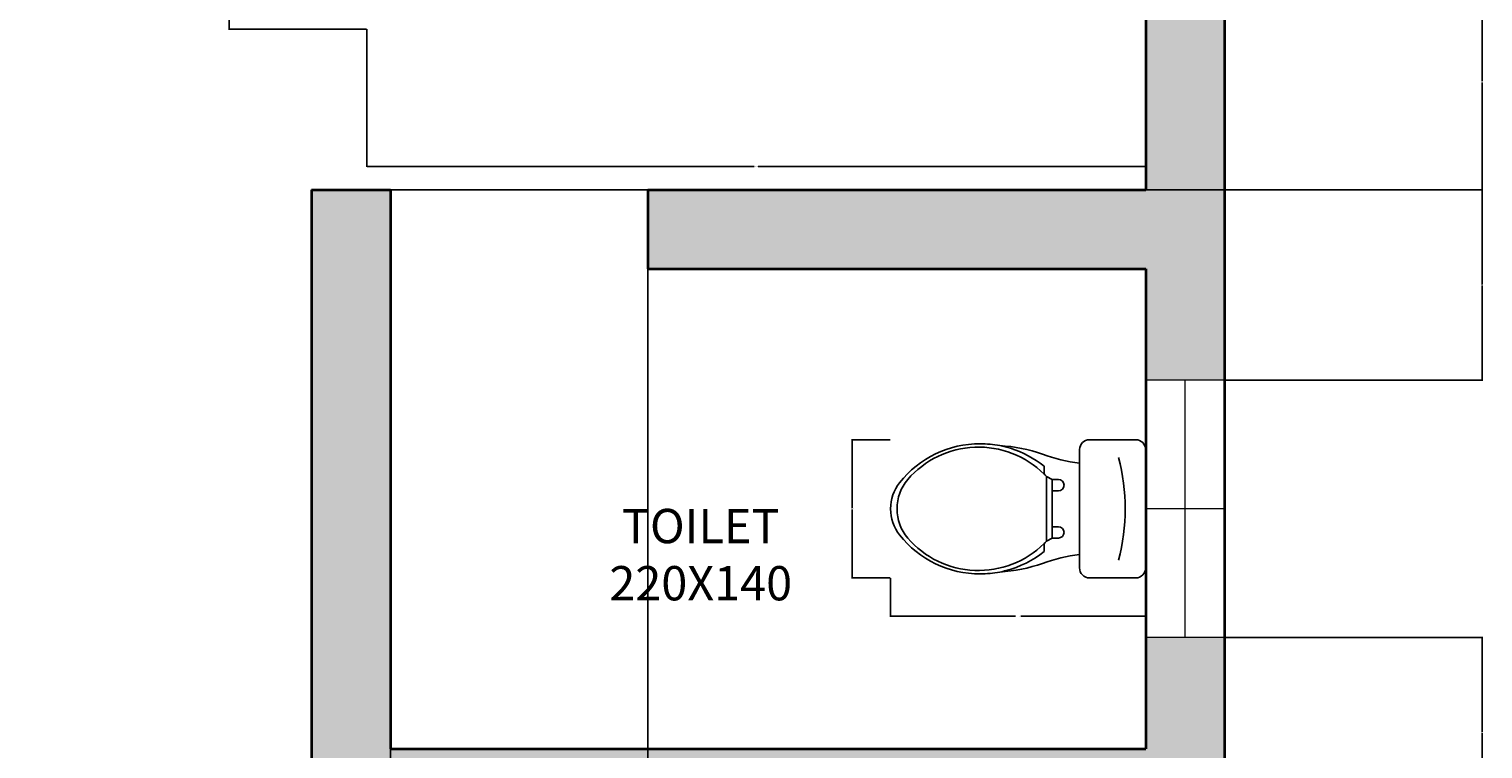
# Model space of a CAD drawing. Units: centimetres. Extents: x 2178 to 3635, y 1064 to 2635.
# Tile 7 of 9: x 3211 to 3635, y 1765 to 1974. Entities that reach past the tile are written whole.
import ezdxf

# ---------------------------------------------------------------- set-up
doc = ezdxf.new("R2010")
doc.units = ezdxf.units.CM
for name, color, linetype, lineweight in [('A-ANNO-DIMS', 2, 'Continuous', 18), ('A-AREA-IDEN', 7, 'Continuous', 18), ('A-DOOR', 32, 'Continuous', 25), ('A-FLOR-FIXT', 42, 'Continuous', 18), ('A-GLAZ', 4, 'Continuous', 18), ('A-WALL', 7, 'Continuous', 35)]:
    doc.layers.add(name, color=color, linetype=linetype, lineweight=lineweight)
doc.layers.add('A-WALL-PATT', color=18, linetype='Continuous', lineweight=13, true_color=0x000000)
doc.layers.add('WC-Detail_dwgmodels.com', color=251, linetype='Continuous')
doc.layers.add('WC-Outline_dwgmodels.com', color=250, linetype='Continuous')
doc.styles.get("Standard").update_dxf_attribs({"font": 'arial.ttf'})
doc.dimstyles.get("Standard").update_dxf_attribs({"dimtxt": 0.18, "dimasz": 0.18, "dimexe": 0.18, "dimexo": 0.0625, "dimgap": 0.09, "dimtad": 0, "dimtih": 1, "dimtoh": 1, "dimdec": 4, "dimzin": 0, "dimdsep": 46, "dimtxsty": 'Standard', "dimcen": 0.09, "dimadec": 0, "dimazin": 0, "dimtfac": 1, "dimtdec": 4, "dimtofl": 0, "dimtmove": 0, "dimatfit": 3, "dimfxl": 1, "dimtolj": 1, "dimtzin": 0, "dimarcsym": 0})

# ---------------------------------------------------------------- blocks, each defined once
blk = doc.blocks.new('pan')
at = {"layer": 'WC-Detail_dwgmodels.com'}
for p, q in [((2845.06, 2654.5), (2845.98, 2656.18)), ((2845.98, 2656.18), (2845.98, 2658.01)), ((2849.25, 2656.18), (2845.98, 2656.18)), ((2849.25, 2658.01), (2849.25, 2656.18)), ((2854.51, 2656.18), (2849.25, 2656.18)), ((2854.51, 2656.18), (2859.76, 2656.18)), ((2859.76, 2658.01), (2859.76, 2656.18)), ((2859.76, 2656.18), (2863.04, 2656.18)), ((2863.04, 2656.18), (2863.04, 2658.01)), ((2863.95, 2654.5), (2863.04, 2656.18)), ((2844.36, 2653.82), (2842.09, 2653.82)), ((2854.51, 2654.5), (2845.06, 2654.5)), ((2854.51, 2654.5), (2863.95, 2654.5)), ((2864.65, 2653.82), (2866.93, 2653.82))]:
    blk.add_line(p, q, dxfattribs=at)
for centre, radius, start, end in [((2854.54, 2618.37), 59.08, 90.028, 104.6712), ((2854.48, 2618.37), 59.08, 75.3288, 89.972), ((2847.61, 2658.01), 1.64, 0, 180), ((2861.4, 2658.01), 1.64, 0, 180), ((2863.72, 2634.72), 27.2, 135.3828, 229.2681), ((2865.36, 2635.16), 29.83, 141.274, 162.7649), ((2863.72, 2634.72), 27.2, 133.3236, 135.3828), ((2845.29, 2634.72), 27.2, 310.7319, 44.6172), ((2845.29, 2634.72), 27.2, 44.6172, 46.6764), ((2843.66, 2635.16), 29.83, 14.6482, 38.726), ((2865.36, 2635.16), 29.83, 162.7649, 168.8583), ((2843.66, 2635.16), 29.83, 11.1417, 14.6482), ((2854.36, 2623.84), 12.85, 229.2681, 270.6684), ((2854.66, 2623.84), 12.85, 269.3316, 310.7319)]:
    blk.add_arc(centre, radius, start, end, dxfattribs=at)
at = {"layer": 'WC-Outline_dwgmodels.com'}
for p, q in [((2854.51, 2683.42), (2837.26, 2683.42)), ((2871.75, 2683.42), (2854.51, 2683.42)), ((2834.37, 2680.53), (2834.37, 2667.05)), ((2874.65, 2667.05), (2874.65, 2680.53)), ((2837.26, 2664.16), (2841.21, 2664.16)), ((2841.21, 2664.16), (2854.51, 2664.16)), ((2867.8, 2664.16), (2854.51, 2664.16)), ((2867.8, 2664.16), (2871.75, 2664.16))]:
    blk.add_line(p, q, dxfattribs=at)
for centre, radius, start, end in [((2837.26, 2680.53), 2.89, 90, 180), ((2871.75, 2680.53), 2.89, 360, 90), ((2837.26, 2667.05), 2.89, 180, 270), ((2788.54, 2671.16), 53.13, 340.4442, 352.4299), ((2920.47, 2671.16), 53.13, 187.5701, 199.5558), ((2871.75, 2667.05), 2.89, 270, 0), ((2880.9, 2638.36), 44.88, 160.4442, 176.7189), ((2828.12, 2638.36), 44.88, 3.2811, 19.5558), ((2865.36, 2635.16), 29.83, 168.8583, 179.8559), ((2843.66, 2635.16), 29.83, 0.1441, 11.1417), ((2865.36, 2635.16), 29.83, 179.8559, 231.7417), ((2843.66, 2635.16), 29.83, 308.2583, 0.1441), ((2854.51, 2621.4), 12.31, 231.7417, 269.9885), ((2854.5, 2621.4), 12.31, 270.0115, 308.2583)]:
    blk.add_arc(centre, radius, start, end, dxfattribs=at)
blk = doc.blocks.new('WIN-0750-2LT')
for p, q in [((0, 0), (0, 23)), ((37.5, 0), (37.5, 23)), ((75, 0), (75, 23)), ((0, 11.5), (75, 11.5))]:
    blk.add_line(p, q)
blk = doc.blocks.new('DOOR-0750')
blk.add_line((0, 0), (75, 0))
blk = doc.blocks.new('*D28')
at = {"layer": 'A-ANNO-DIMS', "color": 0, "lineweight": -2, "transparency": 16777216}
for p, q in [((3309.61, 2241.29), (3269.47, 2241.29)), ((3269.65, 2241.11), (3269.65, 2108.05)), ((3269.65, 1974.63), (3269.65, 2107.68)), ((3309.61, 1974.45), (3269.47, 1974.45))]:
    blk.add_line(p, q, dxfattribs=at)
at = {"layer": 'A-ANNO-DIMS', "color": 0, "transparency": 16777216}
for points in [[(3269.62, 2241.11), (3269.68, 2241.11), (3269.65, 2241.29)], [(3269.62, 1974.63), (3269.68, 1974.63), (3269.65, 1974.45)]]:
    blk.add_solid(points, dxfattribs=at)
at = {"layer": 'Defpoints', "color": 0, "transparency": 16777216}
for p in [(3309.68, 2241.29), (3269.65, 1974.45), (3309.68, 1974.45)]:
    blk.add_point(p, dxfattribs=at)
at = {"layer": 'A-ANNO-DIMS', "color": 0, "transparency": 16777216, "insert": (3269.65, 2107.87), "char_height": 0.18, "attachment_point": 5}
blk.add_mtext('\\A1;BED GROUP 267 TYP.', dxfattribs=at)
blk = doc.blocks.new('*D29')
at = {"layer": 'A-ANNO-DIMS', "color": 0, "lineweight": -2, "transparency": 16777216}
for p, q in [((3309.68, 1974.38), (3309.68, 1934.24)), ((3536.6, 1974.38), (3536.6, 1934.24)), ((3309.86, 1934.42), (3422.54, 1934.42)), ((3536.42, 1934.42), (3423.74, 1934.42))]:
    blk.add_line(p, q, dxfattribs=at)
at = {"layer": 'A-ANNO-DIMS', "color": 0, "transparency": 16777216}
for points in [[(3309.86, 1934.45), (3309.86, 1934.39), (3309.68, 1934.42)], [(3536.42, 1934.45), (3536.42, 1934.39), (3536.6, 1934.42)]]:
    blk.add_solid(points, dxfattribs=at)
at = {"layer": 'Defpoints', "color": 0, "transparency": 16777216}
for p in [(3309.68, 1974.45), (3536.6, 1974.45), (3536.6, 1934.42)]:
    blk.add_point(p, dxfattribs=at)
at = {"layer": 'A-ANNO-DIMS', "color": 0, "transparency": 16777216, "insert": (3423.14, 1934.42), "char_height": 0.18, "attachment_point": 5}
blk.add_mtext('\\A1;227 TYP.', dxfattribs=at)
blk = doc.blocks.new('*D30')
at = {"layer": 'A-ANNO-DIMS', "color": 0, "lineweight": -2, "transparency": 16777216}
for p, q in [((3462.28, 1814.39), (3462.28, 1803.12)), ((3536.6, 1814.39), (3536.6, 1803.12)), ((3462.46, 1803.3), (3498.67, 1803.3)), ((3536.42, 1803.3), (3500.22, 1803.3))]:
    blk.add_line(p, q, dxfattribs=at)
at = {"layer": 'A-ANNO-DIMS', "color": 0, "transparency": 16777216}
for points in [[(3462.46, 1803.33), (3462.46, 1803.27), (3462.28, 1803.3)], [(3536.42, 1803.33), (3536.42, 1803.27), (3536.6, 1803.3)]]:
    blk.add_solid(points, dxfattribs=at)
at = {"layer": 'Defpoints', "color": 0, "transparency": 16777216}
for p in [(3462.28, 1814.45), (3536.6, 1814.45), (3536.6, 1803.3)]:
    blk.add_point(p, dxfattribs=at)
at = {"layer": 'A-ANNO-DIMS', "color": 0, "transparency": 16777216, "insert": (3499.44, 1803.3), "char_height": 0.18, "attachment_point": 5}
blk.add_mtext('\\A1;WC 74 TYP.', dxfattribs=at)
blk = doc.blocks.new('*D31')
at = {"layer": 'A-ANNO-DIMS', "color": 0, "lineweight": -2, "transparency": 16777216}
for p, q in [((3462.22, 1854.73), (3450.95, 1854.73)), ((3451.13, 1854.55), (3451.13, 1834.77)), ((3451.13, 1814.63), (3451.13, 1834.41)), ((3462.22, 1814.45), (3450.95, 1814.45))]:
    blk.add_line(p, q, dxfattribs=at)
at = {"layer": 'A-ANNO-DIMS', "color": 0, "transparency": 16777216}
for points in [[(3451.1, 1854.55), (3451.16, 1854.55), (3451.13, 1854.73)], [(3451.1, 1814.63), (3451.16, 1814.63), (3451.13, 1814.45)]]:
    blk.add_solid(points, dxfattribs=at)
at = {"layer": 'Defpoints', "color": 0, "transparency": 16777216}
for p in [(3462.28, 1854.73), (3451.13, 1814.45), (3462.28, 1814.45)]:
    blk.add_point(p, dxfattribs=at)
at = {"layer": 'A-ANNO-DIMS', "color": 0, "transparency": 16777216, "insert": (3451.13, 1834.59), "char_height": 0.18, "attachment_point": 5}
blk.add_mtext('\\A1;40 TYP.', dxfattribs=at)
blk = doc.blocks.new('*D56')
at = {"layer": 'A-ANNO-DIMS', "color": 0, "lineweight": -2, "transparency": 16777216}
for p, q in [((3559.67, 1990.59), (3634.78, 1990.59)), ((3634.6, 1990.41), (3634.6, 1959.27)), ((3634.6, 1927.77), (3634.6, 1958.91)), ((3536.67, 1927.59), (3634.78, 1927.59))]:
    blk.add_line(p, q, dxfattribs=at)
at = {"layer": 'A-ANNO-DIMS', "color": 0, "transparency": 16777216}
for points in [[(3634.57, 1990.41), (3634.63, 1990.41), (3634.6, 1990.59)], [(3634.57, 1927.77), (3634.63, 1927.77), (3634.6, 1927.59)]]:
    blk.add_solid(points, dxfattribs=at)
at = {"layer": 'Defpoints', "color": 0, "transparency": 16777216}
for p in [(3559.6, 1990.59), (3634.6, 1990.59), (3536.6, 1927.59)]:
    blk.add_point(p, dxfattribs=at)
at = {"layer": 'A-ANNO-DIMS', "color": 0, "transparency": 16777216, "insert": (3634.6, 1959.09), "char_height": 0.18, "attachment_point": 5}
blk.add_mtext('\\A1;63', dxfattribs=at)
blk = doc.blocks.new('*D57')
at = {"layer": 'A-ANNO-DIMS', "color": 0, "lineweight": -2, "transparency": 16777216}
for p, q in [((3536.67, 1927.59), (3634.78, 1927.59)), ((3634.6, 1927.41), (3634.6, 1900.02)), ((3634.6, 1872.27), (3634.6, 1899.66)), ((3559.67, 1872.09), (3634.78, 1872.09))]:
    blk.add_line(p, q, dxfattribs=at)
at = {"layer": 'A-ANNO-DIMS', "color": 0, "transparency": 16777216}
for points in [[(3634.57, 1927.41), (3634.63, 1927.41), (3634.6, 1927.59)], [(3634.57, 1872.27), (3634.63, 1872.27), (3634.6, 1872.09)]]:
    blk.add_solid(points, dxfattribs=at)
at = {"layer": 'Defpoints', "color": 0, "transparency": 16777216}
for p in [(3536.6, 1927.59), (3634.6, 1927.59), (3559.6, 1872.09)]:
    blk.add_point(p, dxfattribs=at)
at = {"layer": 'A-ANNO-DIMS', "color": 0, "transparency": 16777216, "insert": (3634.6, 1899.84), "char_height": 0.18, "attachment_point": 5}
blk.add_mtext('\\A1;55.5', dxfattribs=at)
blk = doc.blocks.new('*D58')
at = {"layer": 'A-ANNO-DIMS', "color": 0, "lineweight": -2, "transparency": 16777216}
for p, q in [((3559.67, 1797.09), (3634.78, 1797.09)), ((3634.6, 1796.91), (3634.6, 1769.52)), ((3634.6, 1741.77), (3634.6, 1769.16)), ((3559.67, 1741.59), (3634.78, 1741.59))]:
    blk.add_line(p, q, dxfattribs=at)
at = {"layer": 'A-ANNO-DIMS', "color": 0, "transparency": 16777216}
for points in [[(3634.57, 1796.91), (3634.63, 1796.91), (3634.6, 1797.09)], [(3634.57, 1741.77), (3634.63, 1741.77), (3634.6, 1741.59)]]:
    blk.add_solid(points, dxfattribs=at)
at = {"layer": 'Defpoints', "color": 0, "transparency": 16777216}
for p in [(3559.6, 1797.09), (3634.6, 1797.09), (3559.6, 1741.59)]:
    blk.add_point(p, dxfattribs=at)
at = {"layer": 'A-ANNO-DIMS', "color": 0, "transparency": 16777216, "insert": (3634.6, 1769.34), "char_height": 0.18, "attachment_point": 5}
blk.add_mtext('\\A1;55.5', dxfattribs=at)
blk = doc.blocks.new('*D67')
at = {"layer": 'A-ANNO-DIMS', "color": 0, "lineweight": -2, "transparency": 16777216}
for p, q in [((3316.6, 1927.53), (3316.6, 1113.41)), ((3391.6, 1927.53), (3391.6, 1113.41)), ((3316.78, 1113.59), (3353.89, 1113.59)), ((3391.42, 1113.59), (3354.32, 1113.59))]:
    blk.add_line(p, q, dxfattribs=at)
at = {"layer": 'A-ANNO-DIMS', "color": 0, "transparency": 16777216}
for points in [[(3316.78, 1113.62), (3316.78, 1113.56), (3316.6, 1113.59)], [(3391.42, 1113.62), (3391.42, 1113.56), (3391.6, 1113.59)]]:
    blk.add_solid(points, dxfattribs=at)
at = {"layer": 'Defpoints', "color": 0, "transparency": 16777216}
for p in [(3316.6, 1927.59), (3391.6, 1927.59), (3391.6, 1113.59)]:
    blk.add_point(p, dxfattribs=at)
at = {"layer": 'A-ANNO-DIMS', "color": 0, "transparency": 16777216, "insert": (3354.1, 1113.59), "char_height": 0.18, "attachment_point": 5}
blk.add_mtext('\\A1;75', dxfattribs=at)

msp = doc.modelspace()

# ---------------------------------------------------------------- hatches: boundary and pattern name
at = {"layer": 'A-WALL-PATT'}
h = msp.add_hatch(color=256, dxfattribs=at)
h.dxf.hatch_style = 1
h.paths.add_polyline_path([(2276.605, 2499.59), (2253.605, 2499.59), (2253.605, 2476.59), (2276.605, 2476.59)])
h.paths.add_polyline_path([(2411.605, 2350.59), (2253.605, 2350.59), (2253.605, 2327.59), (2411.605, 2327.59)])
h.paths.add_polyline_path([(2276.605, 2252.59), (2253.605, 2252.59), (2253.605, 2020.59), (2276.605, 2020.59), (2276.605, 2093.59), (2561.605, 2093.59), (2561.605, 2116.59), (2276.605, 2116.59)])
h.paths.add_polyline_path([(2659.605, 1787.59), (2610.616, 1787.59), (2276.605, 1787.59), (2276.605, 1860.59), (2253.605, 1860.59), (2253.605, 1732.09), (2276.605, 1732.09), (2276.605, 1764.59), (2516.605, 1764.59), (2516.605, 1699.59), (2539.605, 1699.59), (2539.605, 1764.59), (2659.605, 1764.59)])
h.paths.add_polyline_path([(2539.605, 1624.59), (2276.605, 1624.59), (2276.605, 1657.09), (2253.605, 1657.09), (2253.605, 1561.59), (2276.605, 1561.59), (2276.605, 1601.59), (2539.605, 1601.59)])
h.paths.add_polyline_path([(2276.605, 1501.59), (2253.605, 1501.59), (2253.605, 1371.59), (2276.605, 1371.59)])
h.paths.add_polyline_path([(2376.605, 1271.59), (2276.605, 1271.59), (2276.605, 1311.59), (2253.605, 1311.59), (2253.605, 1248.59), (2376.605, 1248.59)])
h.paths.add_polyline_path([(2636.605, 1271.59), (2536.605, 1271.59), (2536.605, 1248.59), (2636.605, 1248.59)])
h.paths.add_polyline_path([(2659.605, 1600.59), (2919.605, 1600.59), (2919.605, 1623.59), (2636.605, 1623.59), (2636.605, 1188.59), (2659.605, 1188.59)])
h.paths.add_polyline_path([(2939.605, 1211.59), (2759.605, 1211.59), (2759.605, 1188.59), (2939.605, 1188.59)])
h.paths.add_polyline_path([(3062.605, 1288.59), (3039.605, 1288.59), (3039.605, 1188.59), (3062.605, 1188.59)])
h.paths.add_polyline_path([(3372.605, 1248.59), (3062.605, 1248.59), (3062.605, 1218.59), (3372.605, 1218.59)])
h.paths.add_polyline_path([(3395.605, 1271.59), (3372.605, 1271.59), (3372.605, 1248.59), (3395.605, 1248.59)])
h.paths.add_polyline_path([(3559.605, 1271.59), (3536.605, 1271.59), (3536.605, 1248.59), (3559.605, 1248.59)])
h.paths.add_polyline_path([(3559.605, 1623.59), (3536.605, 1623.59), (3536.605, 1600.59), (3559.605, 1600.59)])
h.paths.add_polyline_path([(3395.605, 1623.59), (3162.605, 1623.59), (3162.605, 1600.59), (3395.605, 1600.59)])
h.paths.add_polyline_path([(3395.605, 1411.59), (3277.1, 1411.59), (3277.1, 1388.59), (3395.605, 1388.59)])
h.paths.add_polyline_path([(3157.1, 1411.59), (3062.605, 1411.59), (3062.605, 1623.59), (3039.605, 1623.59), (3039.605, 1388.59), (3157.1, 1388.59)])
h.paths.add_polyline_path([(3559.605, 1797.09), (3536.605, 1797.09), (3536.605, 1764.59), (3316.605, 1764.59), (3316.605, 1927.59), (3293.605, 1927.59), (3293.605, 1741.59), (3372.605, 1741.59), (3395.605, 1741.59), (3559.605, 1741.59)])
h.paths.add_polyline_path([(3559.605, 1990.59), (3536.605, 1990.59), (3536.605, 1974.446), (3536.605, 1927.59), (3391.605, 1927.59), (3391.605, 1904.59), (3536.605, 1904.59), (3536.605, 1872.09), (3559.605, 1872.09)])
h.paths.add_polyline_path([(3559.605, 2180.59), (3536.605, 2180.59), (3536.605, 2050.59), (3559.605, 2050.59)])
h.paths.add_polyline_path([(3559.605, 2326.59), (3446.105, 2326.59), (3446.105, 2303.59), (3536.605, 2303.59), (3536.605, 2240.59), (3559.605, 2240.59)])
h.paths.add_polyline_path([(3286.105, 2326.59), (3195.605, 2326.59), (3195.605, 2499.59), (3082.605, 2499.59), (3082.605, 2476.59), (3172.605, 2476.59), (3172.605, 2116.59), (2809.605, 2116.59), (2809.605, 2093.59), (3172.605, 2093.59), (3172.605, 1904.59), (3195.605, 1904.59), (3195.605, 2303.59), (3286.105, 2303.59)])
h.paths.add_polyline_path([(2832.605, 2236.59), (2659.605, 2236.59), (2659.605, 2476.59), (2697.105, 2476.59), (2697.105, 2499.59), (2636.605, 2499.59), (2636.605, 2093.59), (2699.605, 2093.59), (2699.605, 2116.59), (2659.605, 2116.59), (2659.605, 2213.59), (2832.605, 2213.59)])
h.paths.add_polyline_path([(2832.605, 2476.59), (2922.605, 2476.59), (2922.605, 2499.59), (2772.105, 2499.59), (2772.105, 2476.59), (2809.605, 2476.59), (2809.605, 2311.59), (2832.605, 2311.59)])

# ---------------------------------------------------------------- linework, layer by layer
at = {"layer": 'A-WALL'}
for p, q in [((3559.605, 2326.59), (3559.605, 1188.59)), ((3536.605, 2303.59), (3536.605, 1927.59)), ((3293.605, 1927.59), (3293.605, 1741.59)), ((3293.605, 1927.59), (3316.605, 1927.59)), ((3316.605, 1927.59), (3316.605, 1764.59)), ((3391.605, 1927.59), (3391.605, 1904.59)), ((3391.605, 1927.59), (3536.605, 1927.59)), ((3391.605, 1904.59), (3536.605, 1904.59)), ((3536.605, 1904.59), (3536.605, 1764.59)), ((3316.605, 1764.59), (3536.605, 1764.59))]:
    msp.add_line(p, q, dxfattribs=at)

# ---------------------------------------------------------------- block references
at = {"layer": 'A-DOOR'}
msp.add_blockref('DOOR-0750', (3316.605, 1927.59), dxfattribs=at)
at = {"layer": 'A-FLOR-FIXT', "rotation": 270}
msp.add_blockref('pan', (853.186, 4689.097), dxfattribs=at)
at = {"layer": 'A-GLAZ', "rotation": 90.0000000000009}
msp.add_blockref('WIN-0750-2LT', (3559.605, 1797.09), dxfattribs=at)

# ---------------------------------------------------------------- texts
at = {"layer": 'A-AREA-IDEN', "insert": (3351.211, 1834.568), "char_height": 10, "attachment_point": 1}
msp.add_mtext_dynamic_manual_height_columns('\\pxqc;TOILET\\P220X140', width=111.5542, gutter_width=12.5, heights=[0], dxfattribs=at)

# ---------------------------------------------------------------- dimensions: what is measured, and where the dimension line sits
at = {"layer": 'A-ANNO-DIMS'}
for base, p1, p2, text, picture, middle in [((3269.649, 1974.446), (3309.675, 2241.286), (3309.675, 1974.446), 'BED GROUP <> TYP.', '*D28', (3269.649, 2107.866)), ((3451.134, 1814.451), (3462.283, 1854.728), (3462.283, 1814.451), '<> TYP.', '*D31', (3451.134, 1834.59))]:
    dim = msp.add_linear_dim(base=base, p1=p1, p2=p2, angle=270, text=text, dimstyle='Standard', override={"dimdec": 0, "dimlfac": 1, "dimrnd": 0, "dimzin": 0, "dimdsep": 46, "dimlunit": 2}, dxfattribs=at)
    dim.commit()
    dim.dimension.update_dxf_attribs({"geometry": picture, "text_midpoint": middle})
for base, p1, p2, override, picture, middle in [((3634.605, 1990.59), (3536.605, 1927.59), (3559.605, 1990.59), {"dimdec": 0, "dimlfac": 1, "dimrnd": 0, "dimzin": 0, "dimdsep": 46, "dimlunit": 2}, '*D56', (3634.605, 1959.09)), ((3634.605, 1927.59), (3559.605, 1872.09), (3536.605, 1927.59), {"dimdec": 1, "dimlfac": 1, "dimrnd": 0, "dimzin": 0, "dimdsep": 46, "dimlunit": 2}, '*D57', (3634.605, 1899.84)), ((3634.605, 1797.09), (3559.605, 1741.59), (3559.605, 1797.09), {"dimdec": 1, "dimlfac": 1, "dimrnd": 0, "dimzin": 0, "dimdsep": 46, "dimlunit": 2}, '*D58', (3634.605, 1769.34))]:
    dim = msp.add_linear_dim(base=base, p1=p1, p2=p2, angle=90, dimstyle='Standard', override=override, dxfattribs=at)
    dim.commit()
    dim.dimension.update_dxf_attribs({"geometry": picture, "text_midpoint": middle})
for base, p1, p2, text, picture, middle in [((3536.605, 1934.42), (3309.675, 1974.446), (3536.605, 1974.446), '<> TYP.', '*D29', (3423.14, 1934.42)), ((3536.605, 1803.303), (3462.283, 1814.451), (3536.605, 1814.451), 'WC <> TYP.', '*D30', (3499.444, 1803.303))]:
    dim = msp.add_linear_dim(base=base, p1=p1, p2=p2, text=text, dimstyle='Standard', override={"dimdec": 0, "dimlfac": 1, "dimrnd": 0, "dimzin": 0, "dimdsep": 46, "dimlunit": 2}, dxfattribs=at)
    dim.commit()
    dim.dimension.update_dxf_attribs({"geometry": picture, "text_midpoint": middle})
dim = msp.add_linear_dim(base=(3391.605, 1113.59), p1=(3316.605, 1927.59), p2=(3391.605, 1927.59), dimstyle='Standard', override={"dimdec": 0, "dimlfac": 1, "dimrnd": 0, "dimzin": 0, "dimdsep": 46, "dimlunit": 2}, dxfattribs=at)
dim.commit()
dim.dimension.update_dxf_attribs({"geometry": '*D67', "text_midpoint": (3354.105, 1113.59)})

doc.saveas('drawing.dxf')
